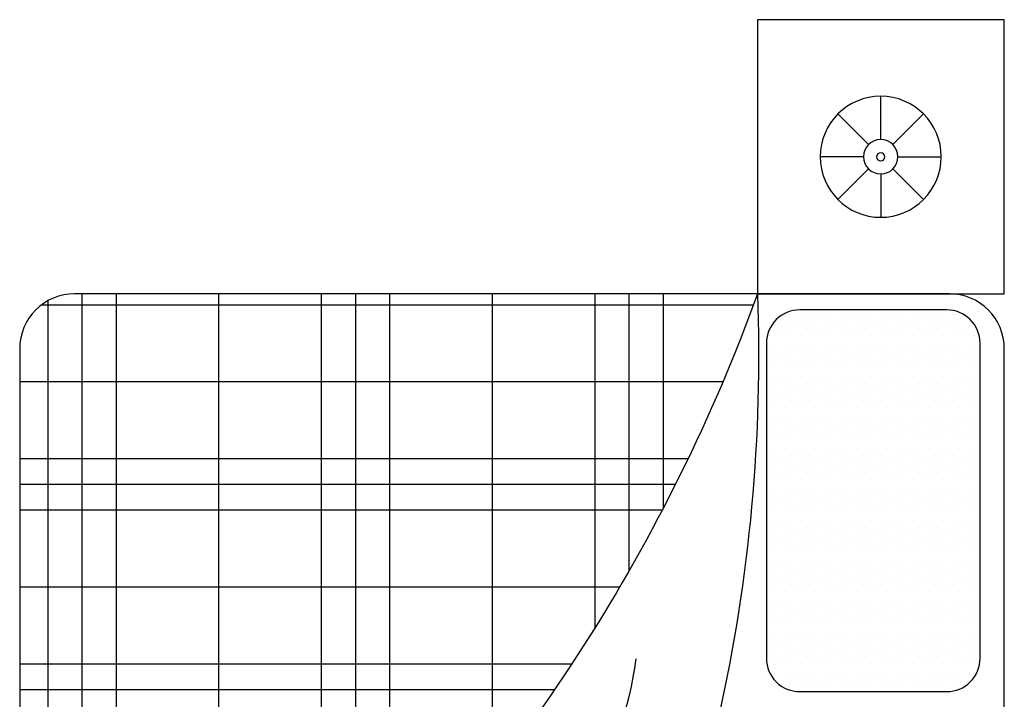
# Model space of a CAD drawing. Units: inches. Extents: x 528 to 2520, y -151 to 1354.
# Tile 39 of 41: x 2385 to 2440, y 770 to 808. Entities that reach past the tile are written whole.
import ezdxf

# ---------------------------------------------------------------- set-up
doc = ezdxf.new("R2010")
doc.units = ezdxf.units.IN
doc.header["$MEASUREMENT"] = 0
doc.layers.add('A-FURN', color=8, linetype='Continuous', lineweight=18)
doc.layers.add('BLOCK', color=6, linetype='Continuous')

# ---------------------------------------------------------------- blocks, each defined once
blk = doc.blocks.new('*X15')
at = {"color": 0}
for p, q in [((276.598, 451.25), (280.51, 451.25)), ((275.455, 450.625), (280.51, 450.625)), ((274.411, 450), (280.51, 450)), ((265.51, 448.125), (267.634, 448.125)), ((271.723, 448.125), (280.51, 448.125)), ((265.51, 446.25), (268.465, 446.25)), ((269.519, 446.25), (280.51, 446.25)), ((265.51, 445.625), (268.531, 445.625)), ((268.866, 445.625), (280.51, 445.625)), ((265.51, 445), (280.51, 445)), ((265.51, 443.125), (280.51, 443.125)), ((265.51, 441.25), (280.51, 441.25)), ((265.51, 440.625), (280.51, 440.625)), ((265.634, 440), (280.386, 440))]:
    blk.add_line(p, q, dxfattribs=at)
blk = doc.blocks.new('*X16')
at = {"color": 0}
for p, q in [((280.312, 439.886), (280.312, 452.896)), ((278.906, 439.482), (278.906, 452.338)), ((277.5, 439.482), (277.5, 451.702)), ((277.031, 439.482), (277.031, 451.471)), ((276.562, 439.482), (276.562, 451.231)), ((275.156, 439.482), (275.156, 450.451)), ((265.781, 439.797), (265.781, 449.511)), ((273.75, 439.482), (273.75, 449.576)), ((266.25, 439.517), (266.25, 449.296)), ((273.281, 439.482), (273.281, 449.261)), ((272.812, 439.482), (272.812, 448.934)), ((267.656, 439.482), (267.656, 448.095)), ((271.406, 439.482), (271.406, 447.876)), ((270, 439.482), (270, 446.689)), ((269.531, 439.482), (269.531, 446.262)), ((269.062, 439.482), (269.062, 445.817))]:
    blk.add_line(p, q, dxfattribs=at)
blk = doc.blocks.new('*X17')
at = {"color": 0}
for p, q in [((273.9375, 457.03125), (273.9375, 457.03125)), ((274.3125, 457.03125), (274.3125, 457.03125)), ((274.6875, 457.03125), (274.6875, 457.03125)), ((275.0625, 457.03125), (275.0625, 457.03125)), ((275.4375, 457.03125), (275.4375, 457.03125)), ((275.8125, 457.03125), (275.8125, 457.03125)), ((276.1875, 457.03125), (276.1875, 457.03125)), ((276.5625, 457.03125), (276.5625, 457.03125)), ((276.9375, 457.03125), (276.9375, 457.03125)), ((277.3125, 457.03125), (277.3125, 457.03125)), ((277.6875, 457.03125), (277.6875, 457.03125)), ((278.0625, 457.03125), (278.0625, 457.03125)), ((278.4375, 457.03125), (278.4375, 457.03125)), ((278.8125, 457.03125), (278.8125, 457.03125)), ((279.1875, 457.03125), (279.1875, 457.03125)), ((279.5625, 457.03125), (279.5625, 457.03125)), ((273.5625, 456.84375), (273.5625, 456.84375)), ((273.75, 456.9375), (273.75, 456.9375)), ((273.9375, 456.84375), (273.9375, 456.84375)), ((274.125, 456.9375), (274.125, 456.9375)), ((274.3125, 456.84375), (274.3125, 456.84375)), ((274.5, 456.9375), (274.5, 456.9375)), ((274.6875, 456.84375), (274.6875, 456.84375)), ((274.875, 456.9375), (274.875, 456.9375)), ((275.0625, 456.84375), (275.0625, 456.84375)), ((275.25, 456.9375), (275.25, 456.9375)), ((275.4375, 456.84375), (275.4375, 456.84375)), ((275.625, 456.9375), (275.625, 456.9375)), ((275.8125, 456.84375), (275.8125, 456.84375)), ((276, 456.9375), (276, 456.9375)), ((276.1875, 456.84375), (276.1875, 456.84375)), ((276.375, 456.9375), (276.375, 456.9375)), ((276.5625, 456.84375), (276.5625, 456.84375)), ((276.75, 456.9375), (276.75, 456.9375)), ((276.9375, 456.84375), (276.9375, 456.84375)), ((277.125, 456.9375), (277.125, 456.9375)), ((277.3125, 456.84375), (277.3125, 456.84375)), ((277.5, 456.9375), (277.5, 456.9375)), ((277.6875, 456.84375), (277.6875, 456.84375)), ((277.875, 456.9375), (277.875, 456.9375)), ((278.0625, 456.84375), (278.0625, 456.84375)), ((278.25, 456.9375), (278.25, 456.9375)), ((278.4375, 456.84375), (278.4375, 456.84375)), ((278.625, 456.9375), (278.625, 456.9375)), ((278.8125, 456.84375), (278.8125, 456.84375)), ((279, 456.9375), (279, 456.9375)), ((279.1875, 456.84375), (279.1875, 456.84375)), ((279.375, 456.9375), (279.375, 456.9375)), ((279.5625, 456.84375), (279.5625, 456.84375)), ((279.75, 456.9375), (279.75, 456.9375)), ((279.9375, 456.84375), (279.9375, 456.84375)), ((273.375, 456.75), (273.375, 456.75)), ((273.75, 456.75), (273.75, 456.75)), ((274.125, 456.75), (274.125, 456.75)), ((274.5, 456.75), (274.5, 456.75)), ((274.875, 456.75), (274.875, 456.75)), ((275.25, 456.75), (275.25, 456.75)), ((275.625, 456.75), (275.625, 456.75)), ((276, 456.75), (276, 456.75)), ((276.375, 456.75), (276.375, 456.75)), ((276.75, 456.75), (276.75, 456.75)), ((277.125, 456.75), (277.125, 456.75)), ((277.5, 456.75), (277.5, 456.75)), ((277.875, 456.75), (277.875, 456.75)), ((278.25, 456.75), (278.25, 456.75)), ((278.625, 456.75), (278.625, 456.75)), ((279, 456.75), (279, 456.75)), ((279.375, 456.75), (279.375, 456.75)), ((279.75, 456.75), (279.75, 456.75)), ((280.125, 456.75), (280.125, 456.75)), ((273.375, 456.5625), (273.375, 456.5625)), ((273.5625, 456.65625), (273.5625, 456.65625)), ((273.75, 456.5625), (273.75, 456.5625)), ((273.9375, 456.65625), (273.9375, 456.65625)), ((274.125, 456.5625), (274.125, 456.5625)), ((274.3125, 456.65625), (274.3125, 456.65625)), ((274.5, 456.5625), (274.5, 456.5625)), ((274.6875, 456.65625), (274.6875, 456.65625)), ((274.875, 456.5625), (274.875, 456.5625)), ((275.0625, 456.65625), (275.0625, 456.65625)), ((275.25, 456.5625), (275.25, 456.5625)), ((275.4375, 456.65625), (275.4375, 456.65625)), ((275.625, 456.5625), (275.625, 456.5625)), ((275.8125, 456.65625), (275.8125, 456.65625)), ((276, 456.5625), (276, 456.5625)), ((276.1875, 456.65625), (276.1875, 456.65625)), ((276.375, 456.5625), (276.375, 456.5625)), ((276.5625, 456.65625), (276.5625, 456.65625)), ((276.75, 456.5625), (276.75, 456.5625)), ((276.9375, 456.65625), (276.9375, 456.65625)), ((277.125, 456.5625), (277.125, 456.5625)), ((277.3125, 456.65625), (277.3125, 456.65625)), ((277.5, 456.5625), (277.5, 456.5625)), ((277.6875, 456.65625), (277.6875, 456.65625)), ((277.875, 456.5625), (277.875, 456.5625)), ((278.0625, 456.65625), (278.0625, 456.65625)), ((278.25, 456.5625), (278.25, 456.5625)), ((278.4375, 456.65625), (278.4375, 456.65625)), ((278.625, 456.5625), (278.625, 456.5625)), ((278.8125, 456.65625), (278.8125, 456.65625)), ((279, 456.5625), (279, 456.5625)), ((279.1875, 456.65625), (279.1875, 456.65625)), ((279.375, 456.5625), (279.375, 456.5625)), ((279.5625, 456.65625), (279.5625, 456.65625)), ((279.75, 456.5625), (279.75, 456.5625)), ((279.9375, 456.65625), (279.9375, 456.65625)), ((280.125, 456.5625), (280.125, 456.5625)), ((273.375, 456.375), (273.375, 456.375)), ((273.5625, 456.46875), (273.5625, 456.46875)), ((273.75, 456.375), (273.75, 456.375)), ((273.9375, 456.46875), (273.9375, 456.46875)), ((274.125, 456.375), (274.125, 456.375)), ((274.3125, 456.46875), (274.3125, 456.46875)), ((274.5, 456.375), (274.5, 456.375)), ((274.6875, 456.46875), (274.6875, 456.46875)), ((274.875, 456.375), (274.875, 456.375)), ((275.0625, 456.46875), (275.0625, 456.46875)), ((275.25, 456.375), (275.25, 456.375)), ((275.4375, 456.46875), (275.4375, 456.46875)), ((275.625, 456.375), (275.625, 456.375)), ((275.8125, 456.46875), (275.8125, 456.46875)), ((276, 456.375), (276, 456.375)), ((276.1875, 456.46875), (276.1875, 456.46875)), ((276.375, 456.375), (276.375, 456.375)), ((276.5625, 456.46875), (276.5625, 456.46875)), ((276.75, 456.375), (276.75, 456.375)), ((276.9375, 456.46875), (276.9375, 456.46875)), ((277.125, 456.375), (277.125, 456.375)), ((277.3125, 456.46875), (277.3125, 456.46875)), ((277.5, 456.375), (277.5, 456.375)), ((277.6875, 456.46875), (277.6875, 456.46875)), ((277.875, 456.375), (277.875, 456.375)), ((278.0625, 456.46875), (278.0625, 456.46875)), ((278.25, 456.375), (278.25, 456.375)), ((278.4375, 456.46875), (278.4375, 456.46875)), ((278.625, 456.375), (278.625, 456.375)), ((278.8125, 456.46875), (278.8125, 456.46875)), ((279, 456.375), (279, 456.375)), ((279.1875, 456.46875), (279.1875, 456.46875)), ((279.375, 456.375), (279.375, 456.375)), ((279.5625, 456.46875), (279.5625, 456.46875)), ((279.75, 456.375), (279.75, 456.375)), ((279.9375, 456.46875), (279.9375, 456.46875)), ((280.125, 456.375), (280.125, 456.375)), ((273.375, 456.1875), (273.375, 456.1875)), ((273.5625, 456.28125), (273.5625, 456.28125)), ((273.75, 456.1875), (273.75, 456.1875)), ((273.9375, 456.28125), (273.9375, 456.28125)), ((274.125, 456.1875), (274.125, 456.1875)), ((274.3125, 456.28125), (274.3125, 456.28125)), ((274.5, 456.1875), (274.5, 456.1875)), ((274.6875, 456.28125), (274.6875, 456.28125)), ((274.875, 456.1875), (274.875, 456.1875)), ((275.0625, 456.28125), (275.0625, 456.28125)), ((275.25, 456.1875), (275.25, 456.1875)), ((275.4375, 456.28125), (275.4375, 456.28125)), ((275.625, 456.1875), (275.625, 456.1875)), ((275.8125, 456.28125), (275.8125, 456.28125)), ((276, 456.1875), (276, 456.1875)), ((276.1875, 456.28125), (276.1875, 456.28125)), ((276.375, 456.1875), (276.375, 456.1875)), ((276.5625, 456.28125), (276.5625, 456.28125)), ((276.75, 456.1875), (276.75, 456.1875)), ((276.9375, 456.28125), (276.9375, 456.28125)), ((277.125, 456.1875), (277.125, 456.1875)), ((277.3125, 456.28125), (277.3125, 456.28125)), ((277.5, 456.1875), (277.5, 456.1875)), ((277.6875, 456.28125), (277.6875, 456.28125)), ((277.875, 456.1875), (277.875, 456.1875)), ((278.0625, 456.28125), (278.0625, 456.28125)), ((278.25, 456.1875), (278.25, 456.1875)), ((278.4375, 456.28125), (278.4375, 456.28125)), ((278.625, 456.1875), (278.625, 456.1875)), ((278.8125, 456.28125), (278.8125, 456.28125)), ((279, 456.1875), (279, 456.1875)), ((279.1875, 456.28125), (279.1875, 456.28125)), ((279.375, 456.1875), (279.375, 456.1875)), ((279.5625, 456.28125), (279.5625, 456.28125)), ((279.75, 456.1875), (279.75, 456.1875)), ((279.9375, 456.28125), (279.9375, 456.28125)), ((280.125, 456.1875), (280.125, 456.1875)), ((273.375, 456), (273.375, 456)), ((273.5625, 456.09375), (273.5625, 456.09375)), ((273.75, 456), (273.75, 456)), ((273.9375, 456.09375), (273.9375, 456.09375)), ((274.125, 456), (274.125, 456)), ((274.3125, 456.09375), (274.3125, 456.09375)), ((274.5, 456), (274.5, 456)), ((274.6875, 456.09375), (274.6875, 456.09375)), ((274.875, 456), (274.875, 456)), ((275.0625, 456.09375), (275.0625, 456.09375)), ((275.25, 456), (275.25, 456)), ((275.4375, 456.09375), (275.4375, 456.09375)), ((275.625, 456), (275.625, 456)), ((275.8125, 456.09375), (275.8125, 456.09375)), ((276, 456), (276, 456)), ((276.1875, 456.09375), (276.1875, 456.09375)), ((276.375, 456), (276.375, 456)), ((276.5625, 456.09375), (276.5625, 456.09375)), ((276.75, 456), (276.75, 456)), ((276.9375, 456.09375), (276.9375, 456.09375)), ((277.125, 456), (277.125, 456)), ((277.3125, 456.09375), (277.3125, 456.09375)), ((277.5, 456), (277.5, 456)), ((277.6875, 456.09375), (277.6875, 456.09375)), ((277.875, 456), (277.875, 456)), ((278.0625, 456.09375), (278.0625, 456.09375)), ((278.25, 456), (278.25, 456)), ((278.4375, 456.09375), (278.4375, 456.09375)), ((278.625, 456), (278.625, 456)), ((278.8125, 456.09375), (278.8125, 456.09375)), ((279, 456), (279, 456)), ((279.1875, 456.09375), (279.1875, 456.09375)), ((279.375, 456), (279.375, 456)), ((279.5625, 456.09375), (279.5625, 456.09375)), ((279.75, 456), (279.75, 456)), ((279.9375, 456.09375), (279.9375, 456.09375)), ((280.125, 456), (280.125, 456)), ((273.375, 455.8125), (273.375, 455.8125)), ((273.5625, 455.90625), (273.5625, 455.90625)), ((273.75, 455.8125), (273.75, 455.8125)), ((273.9375, 455.90625), (273.9375, 455.90625)), ((274.125, 455.8125), (274.125, 455.8125)), ((274.3125, 455.90625), (274.3125, 455.90625)), ((274.5, 455.8125), (274.5, 455.8125)), ((274.6875, 455.90625), (274.6875, 455.90625)), ((274.875, 455.8125), (274.875, 455.8125)), ((275.0625, 455.90625), (275.0625, 455.90625)), ((275.25, 455.8125), (275.25, 455.8125)), ((275.4375, 455.90625), (275.4375, 455.90625)), ((275.625, 455.8125), (275.625, 455.8125)), ((275.8125, 455.90625), (275.8125, 455.90625)), ((276, 455.8125), (276, 455.8125)), ((276.1875, 455.90625), (276.1875, 455.90625)), ((276.375, 455.8125), (276.375, 455.8125)), ((276.5625, 455.90625), (276.5625, 455.90625)), ((276.75, 455.8125), (276.75, 455.8125)), ((276.9375, 455.90625), (276.9375, 455.90625)), ((277.125, 455.8125), (277.125, 455.8125)), ((277.3125, 455.90625), (277.3125, 455.90625)), ((277.5, 455.8125), (277.5, 455.8125)), ((277.6875, 455.90625), (277.6875, 455.90625)), ((277.875, 455.8125), (277.875, 455.8125)), ((278.0625, 455.90625), (278.0625, 455.90625)), ((278.25, 455.8125), (278.25, 455.8125)), ((278.4375, 455.90625), (278.4375, 455.90625)), ((278.625, 455.8125), (278.625, 455.8125)), ((278.8125, 455.90625), (278.8125, 455.90625)), ((279, 455.8125), (279, 455.8125)), ((279.1875, 455.90625), (279.1875, 455.90625)), ((279.375, 455.8125), (279.375, 455.8125)), ((279.5625, 455.90625), (279.5625, 455.90625)), ((279.75, 455.8125), (279.75, 455.8125)), ((279.9375, 455.90625), (279.9375, 455.90625)), ((280.125, 455.8125), (280.125, 455.8125)), ((273.375, 455.625), (273.375, 455.625)), ((273.5625, 455.71875), (273.5625, 455.71875)), ((273.75, 455.625), (273.75, 455.625)), ((273.9375, 455.71875), (273.9375, 455.71875)), ((274.125, 455.625), (274.125, 455.625)), ((274.3125, 455.71875), (274.3125, 455.71875)), ((274.5, 455.625), (274.5, 455.625)), ((274.6875, 455.71875), (274.6875, 455.71875)), ((274.875, 455.625), (274.875, 455.625)), ((275.0625, 455.71875), (275.0625, 455.71875)), ((275.25, 455.625), (275.25, 455.625)), ((275.4375, 455.71875), (275.4375, 455.71875)), ((275.625, 455.625), (275.625, 455.625)), ((275.8125, 455.71875), (275.8125, 455.71875)), ((276, 455.625), (276, 455.625)), ((276.1875, 455.71875), (276.1875, 455.71875)), ((276.375, 455.625), (276.375, 455.625)), ((276.5625, 455.71875), (276.5625, 455.71875)), ((276.75, 455.625), (276.75, 455.625)), ((276.9375, 455.71875), (276.9375, 455.71875)), ((277.125, 455.625), (277.125, 455.625)), ((277.3125, 455.71875), (277.3125, 455.71875)), ((277.5, 455.625), (277.5, 455.625)), ((277.6875, 455.71875), (277.6875, 455.71875)), ((277.875, 455.625), (277.875, 455.625)), ((278.0625, 455.71875), (278.0625, 455.71875)), ((278.25, 455.625), (278.25, 455.625)), ((278.4375, 455.71875), (278.4375, 455.71875)), ((278.625, 455.625), (278.625, 455.625)), ((278.8125, 455.71875), (278.8125, 455.71875)), ((279, 455.625), (279, 455.625)), ((279.1875, 455.71875), (279.1875, 455.71875)), ((279.375, 455.625), (279.375, 455.625)), ((279.5625, 455.71875), (279.5625, 455.71875)), ((279.75, 455.625), (279.75, 455.625)), ((279.9375, 455.71875), (279.9375, 455.71875)), ((280.125, 455.625), (280.125, 455.625)), ((273.375, 455.4375), (273.375, 455.4375)), ((273.5625, 455.53125), (273.5625, 455.53125)), ((273.75, 455.4375), (273.75, 455.4375)), ((273.9375, 455.53125), (273.9375, 455.53125)), ((274.125, 455.4375), (274.125, 455.4375)), ((274.3125, 455.53125), (274.3125, 455.53125)), ((274.5, 455.4375), (274.5, 455.4375)), ((274.6875, 455.53125), (274.6875, 455.53125)), ((274.875, 455.4375), (274.875, 455.4375)), ((275.0625, 455.53125), (275.0625, 455.53125)), ((275.25, 455.4375), (275.25, 455.4375)), ((275.4375, 455.53125), (275.4375, 455.53125)), ((275.625, 455.4375), (275.625, 455.4375)), ((275.8125, 455.53125), (275.8125, 455.53125)), ((276, 455.4375), (276, 455.4375)), ((276.1875, 455.53125), (276.1875, 455.53125)), ((276.375, 455.4375), (276.375, 455.4375)), ((276.5625, 455.53125), (276.5625, 455.53125)), ((276.75, 455.4375), (276.75, 455.4375)), ((276.9375, 455.53125), (276.9375, 455.53125)), ((277.125, 455.4375), (277.125, 455.4375)), ((277.3125, 455.53125), (277.3125, 455.53125)), ((277.5, 455.4375), (277.5, 455.4375)), ((277.6875, 455.53125), (277.6875, 455.53125)), ((277.875, 455.4375), (277.875, 455.4375)), ((278.0625, 455.53125), (278.0625, 455.53125)), ((278.25, 455.4375), (278.25, 455.4375)), ((278.4375, 455.53125), (278.4375, 455.53125)), ((278.625, 455.4375), (278.625, 455.4375)), ((278.8125, 455.53125), (278.8125, 455.53125)), ((279, 455.4375), (279, 455.4375)), ((279.1875, 455.53125), (279.1875, 455.53125)), ((279.375, 455.4375), (279.375, 455.4375)), ((279.5625, 455.53125), (279.5625, 455.53125)), ((279.75, 455.4375), (279.75, 455.4375)), ((279.9375, 455.53125), (279.9375, 455.53125)), ((280.125, 455.4375), (280.125, 455.4375)), ((273.375, 455.25), (273.375, 455.25)), ((273.5625, 455.34375), (273.5625, 455.34375)), ((273.75, 455.25), (273.75, 455.25)), ((273.9375, 455.34375), (273.9375, 455.34375)), ((274.125, 455.25), (274.125, 455.25)), ((274.3125, 455.34375), (274.3125, 455.34375)), ((274.5, 455.25), (274.5, 455.25)), ((274.6875, 455.34375), (274.6875, 455.34375)), ((274.875, 455.25), (274.875, 455.25)), ((275.0625, 455.34375), (275.0625, 455.34375)), ((275.25, 455.25), (275.25, 455.25)), ((275.4375, 455.34375), (275.4375, 455.34375)), ((275.625, 455.25), (275.625, 455.25)), ((275.8125, 455.34375), (275.8125, 455.34375)), ((276, 455.25), (276, 455.25)), ((276.1875, 455.34375), (276.1875, 455.34375)), ((276.375, 455.25), (276.375, 455.25)), ((276.5625, 455.34375), (276.5625, 455.34375)), ((276.75, 455.25), (276.75, 455.25)), ((276.9375, 455.34375), (276.9375, 455.34375)), ((277.125, 455.25), (277.125, 455.25)), ((277.3125, 455.34375), (277.3125, 455.34375)), ((277.5, 455.25), (277.5, 455.25)), ((277.6875, 455.34375), (277.6875, 455.34375)), ((277.875, 455.25), (277.875, 455.25)), ((278.0625, 455.34375), (278.0625, 455.34375)), ((278.25, 455.25), (278.25, 455.25)), ((278.4375, 455.34375), (278.4375, 455.34375)), ((278.625, 455.25), (278.625, 455.25)), ((278.8125, 455.34375), (278.8125, 455.34375)), ((279, 455.25), (279, 455.25)), ((279.1875, 455.34375), (279.1875, 455.34375)), ((279.375, 455.25), (279.375, 455.25)), ((279.5625, 455.34375), (279.5625, 455.34375)), ((279.75, 455.25), (279.75, 455.25)), ((279.9375, 455.34375), (279.9375, 455.34375)), ((280.125, 455.25), (280.125, 455.25)), ((273.375, 455.0625), (273.375, 455.0625)), ((273.5625, 455.15625), (273.5625, 455.15625)), ((273.75, 455.0625), (273.75, 455.0625)), ((273.9375, 455.15625), (273.9375, 455.15625)), ((274.125, 455.0625), (274.125, 455.0625)), ((274.3125, 455.15625), (274.3125, 455.15625)), ((274.5, 455.0625), (274.5, 455.0625)), ((274.6875, 455.15625), (274.6875, 455.15625)), ((274.875, 455.0625), (274.875, 455.0625)), ((275.0625, 455.15625), (275.0625, 455.15625)), ((275.25, 455.0625), (275.25, 455.0625)), ((275.4375, 455.15625), (275.4375, 455.15625)), ((275.625, 455.0625), (275.625, 455.0625)), ((275.8125, 455.15625), (275.8125, 455.15625)), ((276, 455.0625), (276, 455.0625)), ((276.1875, 455.15625), (276.1875, 455.15625)), ((276.375, 455.0625), (276.375, 455.0625)), ((276.5625, 455.15625), (276.5625, 455.15625)), ((276.75, 455.0625), (276.75, 455.0625)), ((276.9375, 455.15625), (276.9375, 455.15625)), ((277.125, 455.0625), (277.125, 455.0625)), ((277.3125, 455.15625), (277.3125, 455.15625)), ((277.5, 455.0625), (277.5, 455.0625)), ((277.6875, 455.15625), (277.6875, 455.15625)), ((277.875, 455.0625), (277.875, 455.0625)), ((278.0625, 455.15625), (278.0625, 455.15625)), ((278.25, 455.0625), (278.25, 455.0625)), ((278.4375, 455.15625), (278.4375, 455.15625)), ((278.625, 455.0625), (278.625, 455.0625)), ((278.8125, 455.15625), (278.8125, 455.15625)), ((279, 455.0625), (279, 455.0625)), ((279.1875, 455.15625), (279.1875, 455.15625)), ((279.375, 455.0625), (279.375, 455.0625)), ((279.5625, 455.15625), (279.5625, 455.15625)), ((279.75, 455.0625), (279.75, 455.0625)), ((279.9375, 455.15625), (279.9375, 455.15625)), ((280.125, 455.0625), (280.125, 455.0625)), ((273.375, 454.875), (273.375, 454.875)), ((273.5625, 454.96875), (273.5625, 454.96875)), ((273.75, 454.875), (273.75, 454.875)), ((273.9375, 454.96875), (273.9375, 454.96875)), ((274.125, 454.875), (274.125, 454.875)), ((274.3125, 454.96875), (274.3125, 454.96875)), ((274.5, 454.875), (274.5, 454.875)), ((274.6875, 454.96875), (274.6875, 454.96875)), ((274.875, 454.875), (274.875, 454.875)), ((275.0625, 454.96875), (275.0625, 454.96875)), ((275.25, 454.875), (275.25, 454.875)), ((275.4375, 454.96875), (275.4375, 454.96875)), ((275.625, 454.875), (275.625, 454.875)), ((275.8125, 454.96875), (275.8125, 454.96875)), ((276, 454.875), (276, 454.875)), ((276.1875, 454.96875), (276.1875, 454.96875)), ((276.375, 454.875), (276.375, 454.875)), ((276.5625, 454.96875), (276.5625, 454.96875)), ((276.75, 454.875), (276.75, 454.875)), ((276.9375, 454.96875), (276.9375, 454.96875)), ((277.125, 454.875), (277.125, 454.875)), ((277.3125, 454.96875), (277.3125, 454.96875)), ((277.5, 454.875), (277.5, 454.875)), ((277.6875, 454.96875), (277.6875, 454.96875)), ((277.875, 454.875), (277.875, 454.875)), ((278.0625, 454.96875), (278.0625, 454.96875)), ((278.25, 454.875), (278.25, 454.875)), ((278.4375, 454.96875), (278.4375, 454.96875)), ((278.625, 454.875), (278.625, 454.875)), ((278.8125, 454.96875), (278.8125, 454.96875)), ((279, 454.875), (279, 454.875)), ((279.1875, 454.96875), (279.1875, 454.96875)), ((279.375, 454.875), (279.375, 454.875)), ((279.5625, 454.96875), (279.5625, 454.96875)), ((279.75, 454.875), (279.75, 454.875)), ((279.9375, 454.96875), (279.9375, 454.96875)), ((280.125, 454.875), (280.125, 454.875)), ((273.375, 454.6875), (273.375, 454.6875)), ((273.5625, 454.78125), (273.5625, 454.78125)), ((273.75, 454.6875), (273.75, 454.6875)), ((273.9375, 454.78125), (273.9375, 454.78125)), ((274.125, 454.6875), (274.125, 454.6875)), ((274.3125, 454.78125), (274.3125, 454.78125)), ((274.5, 454.6875), (274.5, 454.6875)), ((274.6875, 454.78125), (274.6875, 454.78125)), ((274.875, 454.6875), (274.875, 454.6875)), ((275.0625, 454.78125), (275.0625, 454.78125)), ((275.25, 454.6875), (275.25, 454.6875)), ((275.4375, 454.78125), (275.4375, 454.78125)), ((275.625, 454.6875), (275.625, 454.6875)), ((275.8125, 454.78125), (275.8125, 454.78125)), ((276, 454.6875), (276, 454.6875)), ((276.1875, 454.78125), (276.1875, 454.78125)), ((276.375, 454.6875), (276.375, 454.6875)), ((276.5625, 454.78125), (276.5625, 454.78125)), ((276.75, 454.6875), (276.75, 454.6875)), ((276.9375, 454.78125), (276.9375, 454.78125)), ((277.125, 454.6875), (277.125, 454.6875)), ((277.3125, 454.78125), (277.3125, 454.78125)), ((277.5, 454.6875), (277.5, 454.6875)), ((277.6875, 454.78125), (277.6875, 454.78125)), ((277.875, 454.6875), (277.875, 454.6875)), ((278.0625, 454.78125), (278.0625, 454.78125)), ((278.25, 454.6875), (278.25, 454.6875)), ((278.4375, 454.78125), (278.4375, 454.78125)), ((278.625, 454.6875), (278.625, 454.6875)), ((278.8125, 454.78125), (278.8125, 454.78125)), ((279, 454.6875), (279, 454.6875)), ((279.1875, 454.78125), (279.1875, 454.78125)), ((279.375, 454.6875), (279.375, 454.6875)), ((279.5625, 454.78125), (279.5625, 454.78125)), ((279.75, 454.6875), (279.75, 454.6875)), ((279.9375, 454.78125), (279.9375, 454.78125)), ((280.125, 454.6875), (280.125, 454.6875)), ((273.5625, 454.59375), (273.5625, 454.59375)), ((273.9375, 454.59375), (273.9375, 454.59375)), ((274.3125, 454.59375), (274.3125, 454.59375)), ((274.6875, 454.59375), (274.6875, 454.59375)), ((275.0625, 454.59375), (275.0625, 454.59375)), ((275.4375, 454.59375), (275.4375, 454.59375)), ((275.8125, 454.59375), (275.8125, 454.59375)), ((276.1875, 454.59375), (276.1875, 454.59375)), ((276.5625, 454.59375), (276.5625, 454.59375)), ((276.9375, 454.59375), (276.9375, 454.59375)), ((277.3125, 454.59375), (277.3125, 454.59375)), ((277.6875, 454.59375), (277.6875, 454.59375)), ((278.0625, 454.59375), (278.0625, 454.59375)), ((278.4375, 454.59375), (278.4375, 454.59375)), ((278.8125, 454.59375), (278.8125, 454.59375)), ((279.1875, 454.59375), (279.1875, 454.59375)), ((279.5625, 454.59375), (279.5625, 454.59375)), ((279.9375, 454.59375), (279.9375, 454.59375)), ((273.375, 454.5), (273.375, 454.5)), ((273.5625, 454.40625), (273.5625, 454.40625)), ((273.75, 454.5), (273.75, 454.5)), ((273.9375, 454.40625), (273.9375, 454.40625)), ((274.125, 454.5), (274.125, 454.5)), ((274.3125, 454.40625), (274.3125, 454.40625)), ((274.5, 454.5), (274.5, 454.5)), ((274.6875, 454.40625), (274.6875, 454.40625)), ((274.875, 454.5), (274.875, 454.5)), ((275.0625, 454.40625), (275.0625, 454.40625)), ((275.25, 454.5), (275.25, 454.5)), ((275.4375, 454.40625), (275.4375, 454.40625)), ((275.625, 454.5), (275.625, 454.5)), ((275.8125, 454.40625), (275.8125, 454.40625)), ((276, 454.5), (276, 454.5)), ((276.1875, 454.40625), (276.1875, 454.40625)), ((276.375, 454.5), (276.375, 454.5)), ((276.5625, 454.40625), (276.5625, 454.40625)), ((276.75, 454.5), (276.75, 454.5)), ((276.9375, 454.40625), (276.9375, 454.40625)), ((277.125, 454.5), (277.125, 454.5)), ((277.3125, 454.40625), (277.3125, 454.40625)), ((277.5, 454.5), (277.5, 454.5)), ((277.6875, 454.40625), (277.6875, 454.40625)), ((277.875, 454.5), (277.875, 454.5)), ((278.0625, 454.40625), (278.0625, 454.40625)), ((278.25, 454.5), (278.25, 454.5)), ((278.4375, 454.40625), (278.4375, 454.40625)), ((278.625, 454.5), (278.625, 454.5)), ((278.8125, 454.40625), (278.8125, 454.40625)), ((279, 454.5), (279, 454.5)), ((279.1875, 454.40625), (279.1875, 454.40625)), ((279.375, 454.5), (279.375, 454.5)), ((279.5625, 454.40625), (279.5625, 454.40625)), ((279.75, 454.5), (279.75, 454.5)), ((279.9375, 454.40625), (279.9375, 454.40625)), ((280.125, 454.5), (280.125, 454.5)), ((273.375, 454.3125), (273.375, 454.3125)), ((273.5625, 454.21875), (273.5625, 454.21875)), ((273.75, 454.3125), (273.75, 454.3125)), ((273.9375, 454.21875), (273.9375, 454.21875)), ((274.125, 454.3125), (274.125, 454.3125)), ((274.3125, 454.21875), (274.3125, 454.21875)), ((274.5, 454.3125), (274.5, 454.3125)), ((274.6875, 454.21875), (274.6875, 454.21875)), ((274.875, 454.3125), (274.875, 454.3125)), ((275.0625, 454.21875), (275.0625, 454.21875)), ((275.25, 454.3125), (275.25, 454.3125)), ((275.4375, 454.21875), (275.4375, 454.21875)), ((275.625, 454.3125), (275.625, 454.3125)), ((275.8125, 454.21875), (275.8125, 454.21875)), ((276, 454.3125), (276, 454.3125)), ((276.1875, 454.21875), (276.1875, 454.21875)), ((276.375, 454.3125), (276.375, 454.3125)), ((276.5625, 454.21875), (276.5625, 454.21875)), ((276.75, 454.3125), (276.75, 454.3125)), ((276.9375, 454.21875), (276.9375, 454.21875)), ((277.125, 454.3125), (277.125, 454.3125)), ((277.3125, 454.21875), (277.3125, 454.21875)), ((277.5, 454.3125), (277.5, 454.3125)), ((277.6875, 454.21875), (277.6875, 454.21875)), ((277.875, 454.3125), (277.875, 454.3125)), ((278.0625, 454.21875), (278.0625, 454.21875)), ((278.25, 454.3125), (278.25, 454.3125)), ((278.4375, 454.21875), (278.4375, 454.21875)), ((278.625, 454.3125), (278.625, 454.3125)), ((278.8125, 454.21875), (278.8125, 454.21875)), ((279, 454.3125), (279, 454.3125)), ((279.1875, 454.21875), (279.1875, 454.21875)), ((279.375, 454.3125), (279.375, 454.3125)), ((279.5625, 454.21875), (279.5625, 454.21875)), ((279.75, 454.3125), (279.75, 454.3125)), ((279.9375, 454.21875), (279.9375, 454.21875)), ((280.125, 454.3125), (280.125, 454.3125)), ((273.375, 454.125), (273.375, 454.125)), ((273.5625, 454.03125), (273.5625, 454.03125)), ((273.75, 454.125), (273.75, 454.125)), ((273.9375, 454.03125), (273.9375, 454.03125)), ((274.125, 454.125), (274.125, 454.125)), ((274.3125, 454.03125), (274.3125, 454.03125)), ((274.5, 454.125), (274.5, 454.125)), ((274.6875, 454.03125), (274.6875, 454.03125)), ((274.875, 454.125), (274.875, 454.125)), ((275.0625, 454.03125), (275.0625, 454.03125)), ((275.25, 454.125), (275.25, 454.125)), ((275.4375, 454.03125), (275.4375, 454.03125)), ((275.625, 454.125), (275.625, 454.125)), ((275.8125, 454.03125), (275.8125, 454.03125)), ((276, 454.125), (276, 454.125)), ((276.1875, 454.03125), (276.1875, 454.03125)), ((276.375, 454.125), (276.375, 454.125)), ((276.5625, 454.03125), (276.5625, 454.03125)), ((276.75, 454.125), (276.75, 454.125)), ((276.9375, 454.03125), (276.9375, 454.03125)), ((277.125, 454.125), (277.125, 454.125)), ((277.3125, 454.03125), (277.3125, 454.03125)), ((277.5, 454.125), (277.5, 454.125)), ((277.6875, 454.03125), (277.6875, 454.03125)), ((277.875, 454.125), (277.875, 454.125)), ((278.0625, 454.03125), (278.0625, 454.03125)), ((278.25, 454.125), (278.25, 454.125)), ((278.4375, 454.03125), (278.4375, 454.03125)), ((278.625, 454.125), (278.625, 454.125)), ((278.8125, 454.03125), (278.8125, 454.03125)), ((279, 454.125), (279, 454.125)), ((279.1875, 454.03125), (279.1875, 454.03125)), ((279.375, 454.125), (279.375, 454.125)), ((279.5625, 454.03125), (279.5625, 454.03125)), ((279.75, 454.125), (279.75, 454.125)), ((279.9375, 454.03125), (279.9375, 454.03125)), ((280.125, 454.125), (280.125, 454.125)), ((273.375, 453.9375), (273.375, 453.9375)), ((273.5625, 453.84375), (273.5625, 453.84375)), ((273.75, 453.9375), (273.75, 453.9375)), ((273.9375, 453.84375), (273.9375, 453.84375)), ((274.125, 453.9375), (274.125, 453.9375)), ((274.3125, 453.84375), (274.3125, 453.84375)), ((274.5, 453.9375), (274.5, 453.9375)), ((274.6875, 453.84375), (274.6875, 453.84375)), ((274.875, 453.9375), (274.875, 453.9375)), ((275.0625, 453.84375), (275.0625, 453.84375)), ((275.25, 453.9375), (275.25, 453.9375)), ((275.4375, 453.84375), (275.4375, 453.84375)), ((275.625, 453.9375), (275.625, 453.9375)), ((275.8125, 453.84375), (275.8125, 453.84375)), ((276, 453.9375), (276, 453.9375)), ((276.1875, 453.84375), (276.1875, 453.84375)), ((276.375, 453.9375), (276.375, 453.9375)), ((276.5625, 453.84375), (276.5625, 453.84375)), ((276.75, 453.9375), (276.75, 453.9375)), ((276.9375, 453.84375), (276.9375, 453.84375)), ((277.125, 453.9375), (277.125, 453.9375)), ((277.3125, 453.84375), (277.3125, 453.84375)), ((277.5, 453.9375), (277.5, 453.9375)), ((277.6875, 453.84375), (277.6875, 453.84375)), ((277.875, 453.9375), (277.875, 453.9375)), ((278.0625, 453.84375), (278.0625, 453.84375)), ((278.25, 453.9375), (278.25, 453.9375)), ((278.4375, 453.84375), (278.4375, 453.84375)), ((278.625, 453.9375), (278.625, 453.9375)), ((278.8125, 453.84375), (278.8125, 453.84375)), ((279, 453.9375), (279, 453.9375)), ((279.1875, 453.84375), (279.1875, 453.84375)), ((279.375, 453.9375), (279.375, 453.9375)), ((279.5625, 453.84375), (279.5625, 453.84375)), ((279.75, 453.9375), (279.75, 453.9375)), ((279.9375, 453.84375), (279.9375, 453.84375)), ((280.125, 453.9375), (280.125, 453.9375)), ((273.375, 453.75), (273.375, 453.75)), ((273.5625, 453.65625), (273.5625, 453.65625)), ((273.75, 453.75), (273.75, 453.75)), ((273.9375, 453.65625), (273.9375, 453.65625)), ((274.125, 453.75), (274.125, 453.75)), ((274.3125, 453.65625), (274.3125, 453.65625)), ((274.5, 453.75), (274.5, 453.75)), ((274.6875, 453.65625), (274.6875, 453.65625)), ((274.875, 453.75), (274.875, 453.75)), ((275.0625, 453.65625), (275.0625, 453.65625)), ((275.25, 453.75), (275.25, 453.75)), ((275.4375, 453.65625), (275.4375, 453.65625)), ((275.625, 453.75), (275.625, 453.75)), ((275.8125, 453.65625), (275.8125, 453.65625)), ((276, 453.75), (276, 453.75)), ((276.1875, 453.65625), (276.1875, 453.65625)), ((276.375, 453.75), (276.375, 453.75)), ((276.5625, 453.65625), (276.5625, 453.65625)), ((276.75, 453.75), (276.75, 453.75)), ((276.9375, 453.65625), (276.9375, 453.65625)), ((277.125, 453.75), (277.125, 453.75)), ((277.3125, 453.65625), (277.3125, 453.65625)), ((277.5, 453.75), (277.5, 453.75)), ((277.6875, 453.65625), (277.6875, 453.65625)), ((277.875, 453.75), (277.875, 453.75)), ((278.0625, 453.65625), (278.0625, 453.65625)), ((278.25, 453.75), (278.25, 453.75)), ((278.4375, 453.65625), (278.4375, 453.65625)), ((278.625, 453.75), (278.625, 453.75)), ((278.8125, 453.65625), (278.8125, 453.65625)), ((279, 453.75), (279, 453.75)), ((279.1875, 453.65625), (279.1875, 453.65625)), ((279.375, 453.75), (279.375, 453.75)), ((279.5625, 453.65625), (279.5625, 453.65625)), ((279.75, 453.75), (279.75, 453.75)), ((279.9375, 453.65625), (279.9375, 453.65625)), ((280.125, 453.75), (280.125, 453.75)), ((273.375, 453.5625), (273.375, 453.5625)), ((273.5625, 453.46875), (273.5625, 453.46875)), ((273.75, 453.5625), (273.75, 453.5625)), ((273.9375, 453.46875), (273.9375, 453.46875)), ((274.125, 453.5625), (274.125, 453.5625)), ((274.3125, 453.46875), (274.3125, 453.46875)), ((274.5, 453.5625), (274.5, 453.5625)), ((274.6875, 453.46875), (274.6875, 453.46875)), ((274.875, 453.5625), (274.875, 453.5625)), ((275.0625, 453.46875), (275.0625, 453.46875)), ((275.25, 453.5625), (275.25, 453.5625)), ((275.4375, 453.46875), (275.4375, 453.46875)), ((275.625, 453.5625), (275.625, 453.5625)), ((275.8125, 453.46875), (275.8125, 453.46875)), ((276, 453.5625), (276, 453.5625)), ((276.1875, 453.46875), (276.1875, 453.46875)), ((276.375, 453.5625), (276.375, 453.5625)), ((276.5625, 453.46875), (276.5625, 453.46875)), ((276.75, 453.5625), (276.75, 453.5625)), ((276.9375, 453.46875), (276.9375, 453.46875)), ((277.125, 453.5625), (277.125, 453.5625)), ((277.3125, 453.46875), (277.3125, 453.46875)), ((277.5, 453.5625), (277.5, 453.5625)), ((277.6875, 453.46875), (277.6875, 453.46875)), ((277.875, 453.5625), (277.875, 453.5625)), ((278.0625, 453.46875), (278.0625, 453.46875)), ((278.25, 453.5625), (278.25, 453.5625)), ((278.4375, 453.46875), (278.4375, 453.46875)), ((278.625, 453.5625), (278.625, 453.5625)), ((278.8125, 453.46875), (278.8125, 453.46875)), ((279, 453.5625), (279, 453.5625)), ((279.1875, 453.46875), (279.1875, 453.46875)), ((279.375, 453.5625), (279.375, 453.5625)), ((279.5625, 453.46875), (279.5625, 453.46875)), ((279.75, 453.5625), (279.75, 453.5625)), ((279.9375, 453.46875), (279.9375, 453.46875)), ((280.125, 453.5625), (280.125, 453.5625)), ((273.375, 453.375), (273.375, 453.375)), ((273.5625, 453.28125), (273.5625, 453.28125)), ((273.75, 453.375), (273.75, 453.375)), ((273.9375, 453.28125), (273.9375, 453.28125)), ((274.125, 453.375), (274.125, 453.375)), ((274.3125, 453.28125), (274.3125, 453.28125)), ((274.5, 453.375), (274.5, 453.375)), ((274.6875, 453.28125), (274.6875, 453.28125)), ((274.875, 453.375), (274.875, 453.375)), ((275.0625, 453.28125), (275.0625, 453.28125)), ((275.25, 453.375), (275.25, 453.375)), ((275.4375, 453.28125), (275.4375, 453.28125)), ((275.625, 453.375), (275.625, 453.375)), ((275.8125, 453.28125), (275.8125, 453.28125)), ((276, 453.375), (276, 453.375)), ((276.1875, 453.28125), (276.1875, 453.28125)), ((276.375, 453.375), (276.375, 453.375)), ((276.5625, 453.28125), (276.5625, 453.28125)), ((276.75, 453.375), (276.75, 453.375)), ((276.9375, 453.28125), (276.9375, 453.28125)), ((277.125, 453.375), (277.125, 453.375)), ((277.3125, 453.28125), (277.3125, 453.28125)), ((277.5, 453.375), (277.5, 453.375)), ((277.6875, 453.28125), (277.6875, 453.28125)), ((277.875, 453.375), (277.875, 453.375)), ((278.0625, 453.28125), (278.0625, 453.28125)), ((278.25, 453.375), (278.25, 453.375)), ((278.4375, 453.28125), (278.4375, 453.28125)), ((278.625, 453.375), (278.625, 453.375)), ((278.8125, 453.28125), (278.8125, 453.28125)), ((279, 453.375), (279, 453.375)), ((279.1875, 453.28125), (279.1875, 453.28125)), ((279.375, 453.375), (279.375, 453.375)), ((279.5625, 453.28125), (279.5625, 453.28125)), ((279.75, 453.375), (279.75, 453.375)), ((279.9375, 453.28125), (279.9375, 453.28125)), ((273.75, 453.1875), (273.75, 453.1875)), ((274.125, 453.1875), (274.125, 453.1875)), ((274.5, 453.1875), (274.5, 453.1875)), ((274.875, 453.1875), (274.875, 453.1875)), ((275.25, 453.1875), (275.25, 453.1875)), ((275.625, 453.1875), (275.625, 453.1875)), ((276, 453.1875), (276, 453.1875)), ((276.375, 453.1875), (276.375, 453.1875)), ((276.75, 453.1875), (276.75, 453.1875)), ((277.125, 453.1875), (277.125, 453.1875)), ((277.5, 453.1875), (277.5, 453.1875)), ((277.875, 453.1875), (277.875, 453.1875)), ((278.25, 453.1875), (278.25, 453.1875)), ((278.625, 453.1875), (278.625, 453.1875)), ((279, 453.1875), (279, 453.1875)), ((279.375, 453.1875), (279.375, 453.1875)), ((279.75, 453.1875), (279.75, 453.1875))]:
    blk.add_line(p, q, dxfattribs=at)
blk = doc.blocks.new('A$C52E67D0D')
at = {"layer": 'BLOCK'}
for p, q in [((2251.5, 1605.5), (2251.5, 1684.7)), ((2229.3, 1596.3), (2173.3, 1652.3)), ((2273.7, 1596.3), (2329.7, 1652.3)), ((2220.1, 1574.1), (2140.9, 1574.1)), ((2282.9, 1574.1), (2362.1, 1574.1)), ((2229.3, 1551.9), (2173.3, 1495.9)), ((2273.7, 1551.9), (2329.7, 1495.9)), ((2251.5, 1542.8), (2251.5, 1463.5))]:
    blk.add_line(p, q, dxfattribs=at)
for points in [[(1901, 0), (601, 0, -0.414214), (501, 100), (501, 1700, -0.414214), (601, 1800), (1901, 1800, -0.414214), (2001, 1700), (2001, 100, -0.414214)], [(1911, 1365.1), (1335, 1365.1, -0.414214), (1274.2, 1425.9), (1274.2, 1694.8, -0.414214), (1335, 1755.7), (1911, 1755.7, -0.414214), (1971.8, 1694.8), (1971.8, 1425.9, -0.414214)]]:
    blk.add_lwpolyline(points, format="xyb", close=True, dxfattribs=at)
blk.add_lwpolyline([(2001, 1348.6), (2001, 1799.6), (2502, 1799.6), (2502, 1348.6)], close=True, dxfattribs=at)
for radius in [110.6, 31.4, 7.46]:
    blk.add_circle((2251.5, 1574.1), radius, dxfattribs=at)
for centre, radius, start, end in [((1888.6, -1664.5), 3015.3, 87.8642, 117.4001), ((3101, -1685.8), 3227.7, 109.926, 135.3977), ((1410.8, 520.2), 610.8, 97.2157, 147.6656)]:
    blk.add_arc(centre, radius, start, end, dxfattribs=at)
at = {"layer": 'BLOCK', "xscale": 100, "yscale": 100, "zscale": 100}
for name in ['*X17', '*X16', '*X15']:
    blk.add_blockref(name, (-26050, -43948.2), dxfattribs=at)

msp = doc.modelspace()

# ---------------------------------------------------------------- block references
at = {"layer": 'A-FURN', "xscale": -0.0306954436450662, "yscale": 0.0306954436450662, "zscale": 0.0306954436450662, "rotation": 270}
msp.add_blockref('A$C52E67D0D', (2385.117, 731.467), dxfattribs=at)

doc.saveas('drawing.dxf')
